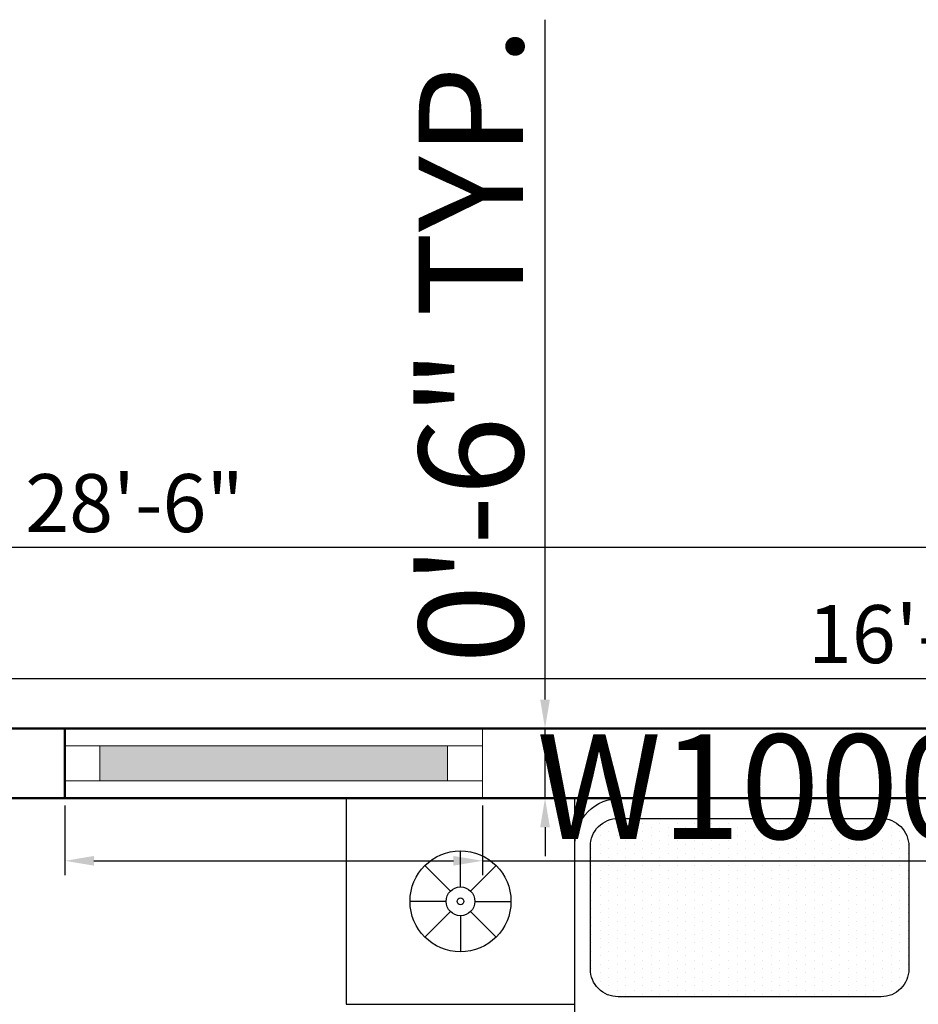
# Model space of a CAD drawing. Units: inches. Extents: x 3064 to 19385, y 846 to 15425.
# Tile 46 of 108: x 5352 to 5430, y 1368 to 1453. Entities that reach past the tile are written whole.
import ezdxf

# ---------------------------------------------------------------- set-up
doc = ezdxf.new("R2010")
doc.units = ezdxf.units.IN
for name, color, linetype, lineweight in [('A-ANNO-DIMS', 2, 'Continuous', 18), ('A-FLOR-FIXT', 9, 'Continuous', 18), ('A-GLAZ', 4, 'Continuous', 18), ('A-WALL', 7, 'Continuous', 50)]:
    doc.layers.add(name, color=color, linetype=linetype, lineweight=lineweight)
doc.layers.add('BLOCK', color=6, linetype='Continuous')
doc.styles.get("Standard").update_dxf_attribs({"font": 'arial.ttf'})
doc.dimstyles.new('ISO-25', dxfattribs={"dimtxt": 9, "dimasz": 2.5, "dimexe": 1.25, "dimexo": 0.625, "dimtad": 1, "dimdec": 1, "dimlunit": 3, "dimtxsty": 'Standard', "dimcen": 2.5, "dimadec": 0, "dimazin": 0, "dimtfac": 1, "dimtdec": 1, "dimtmove": 0, "dimatfit": 3, "dimfxl": 1, "dimarcsym": 0})

# ---------------------------------------------------------------- blocks, each defined once
blk = doc.blocks.new('*X7')
at = {"color": 0}
for p, q in [((266.25, 456.9375), (266.25, 456.9375)), ((266.4375, 457.03125), (266.4375, 457.03125)), ((266.625, 456.9375), (266.625, 456.9375)), ((266.8125, 457.03125), (266.8125, 457.03125)), ((267, 456.9375), (267, 456.9375)), ((267.1875, 457.03125), (267.1875, 457.03125)), ((267.375, 456.9375), (267.375, 456.9375)), ((267.5625, 457.03125), (267.5625, 457.03125)), ((267.75, 456.9375), (267.75, 456.9375)), ((267.9375, 457.03125), (267.9375, 457.03125)), ((268.125, 456.9375), (268.125, 456.9375)), ((268.3125, 457.03125), (268.3125, 457.03125)), ((268.5, 456.9375), (268.5, 456.9375)), ((268.6875, 457.03125), (268.6875, 457.03125)), ((268.875, 456.9375), (268.875, 456.9375)), ((269.0625, 457.03125), (269.0625, 457.03125)), ((269.25, 456.9375), (269.25, 456.9375)), ((269.4375, 457.03125), (269.4375, 457.03125)), ((269.625, 456.9375), (269.625, 456.9375)), ((269.8125, 457.03125), (269.8125, 457.03125)), ((270, 456.9375), (270, 456.9375)), ((270.1875, 457.03125), (270.1875, 457.03125)), ((270.375, 456.9375), (270.375, 456.9375)), ((270.5625, 457.03125), (270.5625, 457.03125)), ((270.75, 456.9375), (270.75, 456.9375)), ((270.9375, 457.03125), (270.9375, 457.03125)), ((271.125, 456.9375), (271.125, 456.9375)), ((271.3125, 457.03125), (271.3125, 457.03125)), ((271.5, 456.9375), (271.5, 456.9375)), ((271.6875, 457.03125), (271.6875, 457.03125)), ((271.875, 456.9375), (271.875, 456.9375)), ((272.0625, 457.03125), (272.0625, 457.03125)), ((272.25, 456.9375), (272.25, 456.9375)), ((266.0625, 456.84375), (266.0625, 456.84375)), ((266.0625, 456.65625), (266.0625, 456.65625)), ((266.25, 456.75), (266.25, 456.75)), ((266.4375, 456.84375), (266.4375, 456.84375)), ((266.4375, 456.65625), (266.4375, 456.65625)), ((266.625, 456.75), (266.625, 456.75)), ((266.8125, 456.84375), (266.8125, 456.84375)), ((266.8125, 456.65625), (266.8125, 456.65625)), ((267, 456.75), (267, 456.75)), ((267.1875, 456.84375), (267.1875, 456.84375)), ((267.1875, 456.65625), (267.1875, 456.65625)), ((267.375, 456.75), (267.375, 456.75)), ((267.5625, 456.84375), (267.5625, 456.84375)), ((267.5625, 456.65625), (267.5625, 456.65625)), ((267.75, 456.75), (267.75, 456.75)), ((267.9375, 456.84375), (267.9375, 456.84375)), ((267.9375, 456.65625), (267.9375, 456.65625)), ((268.125, 456.75), (268.125, 456.75)), ((268.3125, 456.84375), (268.3125, 456.84375)), ((268.3125, 456.65625), (268.3125, 456.65625)), ((268.5, 456.75), (268.5, 456.75)), ((268.6875, 456.84375), (268.6875, 456.84375)), ((268.6875, 456.65625), (268.6875, 456.65625)), ((268.875, 456.75), (268.875, 456.75)), ((269.0625, 456.84375), (269.0625, 456.84375)), ((269.0625, 456.65625), (269.0625, 456.65625)), ((269.25, 456.75), (269.25, 456.75)), ((269.4375, 456.84375), (269.4375, 456.84375)), ((269.4375, 456.65625), (269.4375, 456.65625)), ((269.625, 456.75), (269.625, 456.75)), ((269.8125, 456.84375), (269.8125, 456.84375)), ((269.8125, 456.65625), (269.8125, 456.65625)), ((270, 456.75), (270, 456.75)), ((270.1875, 456.84375), (270.1875, 456.84375)), ((270.1875, 456.65625), (270.1875, 456.65625)), ((270.375, 456.75), (270.375, 456.75)), ((270.5625, 456.84375), (270.5625, 456.84375)), ((270.5625, 456.65625), (270.5625, 456.65625)), ((270.75, 456.75), (270.75, 456.75)), ((270.9375, 456.84375), (270.9375, 456.84375)), ((270.9375, 456.65625), (270.9375, 456.65625)), ((271.125, 456.75), (271.125, 456.75)), ((271.3125, 456.84375), (271.3125, 456.84375)), ((271.3125, 456.65625), (271.3125, 456.65625)), ((271.5, 456.75), (271.5, 456.75)), ((271.6875, 456.84375), (271.6875, 456.84375)), ((271.6875, 456.65625), (271.6875, 456.65625)), ((271.875, 456.75), (271.875, 456.75)), ((272.0625, 456.84375), (272.0625, 456.84375)), ((272.0625, 456.65625), (272.0625, 456.65625)), ((272.25, 456.75), (272.25, 456.75)), ((272.4375, 456.84375), (272.4375, 456.84375)), ((272.4375, 456.65625), (272.4375, 456.65625)), ((272.625, 456.75), (272.625, 456.75)), ((265.875, 456.5625), (265.875, 456.5625)), ((266.0625, 456.46875), (266.0625, 456.46875)), ((266.25, 456.5625), (266.25, 456.5625)), ((266.4375, 456.46875), (266.4375, 456.46875)), ((266.625, 456.5625), (266.625, 456.5625)), ((266.8125, 456.46875), (266.8125, 456.46875)), ((267, 456.5625), (267, 456.5625)), ((267.1875, 456.46875), (267.1875, 456.46875)), ((267.375, 456.5625), (267.375, 456.5625)), ((267.5625, 456.46875), (267.5625, 456.46875)), ((267.75, 456.5625), (267.75, 456.5625)), ((267.9375, 456.46875), (267.9375, 456.46875)), ((268.125, 456.5625), (268.125, 456.5625)), ((268.3125, 456.46875), (268.3125, 456.46875)), ((268.5, 456.5625), (268.5, 456.5625)), ((268.6875, 456.46875), (268.6875, 456.46875)), ((268.875, 456.5625), (268.875, 456.5625)), ((269.0625, 456.46875), (269.0625, 456.46875)), ((269.25, 456.5625), (269.25, 456.5625)), ((269.4375, 456.46875), (269.4375, 456.46875)), ((269.625, 456.5625), (269.625, 456.5625)), ((269.8125, 456.46875), (269.8125, 456.46875)), ((270, 456.5625), (270, 456.5625)), ((270.1875, 456.46875), (270.1875, 456.46875)), ((270.375, 456.5625), (270.375, 456.5625)), ((270.5625, 456.46875), (270.5625, 456.46875)), ((270.75, 456.5625), (270.75, 456.5625)), ((270.9375, 456.46875), (270.9375, 456.46875)), ((271.125, 456.5625), (271.125, 456.5625)), ((271.3125, 456.46875), (271.3125, 456.46875)), ((271.5, 456.5625), (271.5, 456.5625)), ((271.6875, 456.46875), (271.6875, 456.46875)), ((271.875, 456.5625), (271.875, 456.5625)), ((272.0625, 456.46875), (272.0625, 456.46875)), ((272.25, 456.5625), (272.25, 456.5625)), ((272.4375, 456.46875), (272.4375, 456.46875)), ((272.625, 456.5625), (272.625, 456.5625)), ((272.8125, 456.46875), (272.8125, 456.46875)), ((265.875, 456.375), (265.875, 456.375)), ((266.0625, 456.28125), (266.0625, 456.28125)), ((266.25, 456.375), (266.25, 456.375)), ((266.4375, 456.28125), (266.4375, 456.28125)), ((266.625, 456.375), (266.625, 456.375)), ((266.8125, 456.28125), (266.8125, 456.28125)), ((267, 456.375), (267, 456.375)), ((267.1875, 456.28125), (267.1875, 456.28125)), ((267.375, 456.375), (267.375, 456.375)), ((267.5625, 456.28125), (267.5625, 456.28125)), ((267.75, 456.375), (267.75, 456.375)), ((267.9375, 456.28125), (267.9375, 456.28125)), ((268.125, 456.375), (268.125, 456.375)), ((268.3125, 456.28125), (268.3125, 456.28125)), ((268.5, 456.375), (268.5, 456.375)), ((268.6875, 456.28125), (268.6875, 456.28125)), ((268.875, 456.375), (268.875, 456.375)), ((269.0625, 456.28125), (269.0625, 456.28125)), ((269.25, 456.375), (269.25, 456.375)), ((269.4375, 456.28125), (269.4375, 456.28125)), ((269.625, 456.375), (269.625, 456.375)), ((269.8125, 456.28125), (269.8125, 456.28125)), ((270, 456.375), (270, 456.375)), ((270.1875, 456.28125), (270.1875, 456.28125)), ((270.375, 456.375), (270.375, 456.375)), ((270.5625, 456.28125), (270.5625, 456.28125)), ((270.75, 456.375), (270.75, 456.375)), ((270.9375, 456.28125), (270.9375, 456.28125)), ((271.125, 456.375), (271.125, 456.375)), ((271.3125, 456.28125), (271.3125, 456.28125)), ((271.5, 456.375), (271.5, 456.375)), ((271.6875, 456.28125), (271.6875, 456.28125)), ((271.875, 456.375), (271.875, 456.375)), ((272.0625, 456.28125), (272.0625, 456.28125)), ((272.25, 456.375), (272.25, 456.375)), ((272.4375, 456.28125), (272.4375, 456.28125)), ((272.625, 456.375), (272.625, 456.375)), ((272.8125, 456.28125), (272.8125, 456.28125)), ((265.875, 456.1875), (265.875, 456.1875)), ((265.875, 456), (265.875, 456)), ((266.0625, 456.09375), (266.0625, 456.09375)), ((266.25, 456.1875), (266.25, 456.1875)), ((266.25, 456), (266.25, 456)), ((266.4375, 456.09375), (266.4375, 456.09375)), ((266.625, 456.1875), (266.625, 456.1875)), ((266.625, 456), (266.625, 456)), ((266.8125, 456.09375), (266.8125, 456.09375)), ((267, 456.1875), (267, 456.1875)), ((267, 456), (267, 456)), ((267.1875, 456.09375), (267.1875, 456.09375)), ((267.375, 456.1875), (267.375, 456.1875)), ((267.375, 456), (267.375, 456)), ((267.5625, 456.09375), (267.5625, 456.09375)), ((267.75, 456.1875), (267.75, 456.1875)), ((267.75, 456), (267.75, 456)), ((267.9375, 456.09375), (267.9375, 456.09375)), ((268.125, 456.1875), (268.125, 456.1875)), ((268.125, 456), (268.125, 456)), ((268.3125, 456.09375), (268.3125, 456.09375)), ((268.5, 456.1875), (268.5, 456.1875)), ((268.5, 456), (268.5, 456)), ((268.6875, 456.09375), (268.6875, 456.09375)), ((268.875, 456.1875), (268.875, 456.1875)), ((268.875, 456), (268.875, 456)), ((269.0625, 456.09375), (269.0625, 456.09375)), ((269.25, 456.1875), (269.25, 456.1875)), ((269.25, 456), (269.25, 456)), ((269.4375, 456.09375), (269.4375, 456.09375)), ((269.625, 456.1875), (269.625, 456.1875)), ((269.625, 456), (269.625, 456)), ((269.8125, 456.09375), (269.8125, 456.09375)), ((270, 456.1875), (270, 456.1875)), ((270, 456), (270, 456)), ((270.1875, 456.09375), (270.1875, 456.09375)), ((270.375, 456.1875), (270.375, 456.1875)), ((270.375, 456), (270.375, 456)), ((270.5625, 456.09375), (270.5625, 456.09375)), ((270.75, 456.1875), (270.75, 456.1875)), ((270.75, 456), (270.75, 456)), ((270.9375, 456.09375), (270.9375, 456.09375)), ((271.125, 456.1875), (271.125, 456.1875)), ((271.125, 456), (271.125, 456)), ((271.3125, 456.09375), (271.3125, 456.09375)), ((271.5, 456.1875), (271.5, 456.1875)), ((271.5, 456), (271.5, 456)), ((271.6875, 456.09375), (271.6875, 456.09375)), ((271.875, 456.1875), (271.875, 456.1875)), ((271.875, 456), (271.875, 456)), ((272.0625, 456.09375), (272.0625, 456.09375)), ((272.25, 456.1875), (272.25, 456.1875)), ((272.25, 456), (272.25, 456)), ((272.4375, 456.09375), (272.4375, 456.09375)), ((272.625, 456.1875), (272.625, 456.1875)), ((272.625, 456), (272.625, 456)), ((272.8125, 456.09375), (272.8125, 456.09375)), ((265.875, 455.8125), (265.875, 455.8125)), ((266.0625, 455.90625), (266.0625, 455.90625)), ((266.25, 455.8125), (266.25, 455.8125)), ((266.4375, 455.90625), (266.4375, 455.90625)), ((266.625, 455.8125), (266.625, 455.8125)), ((266.8125, 455.90625), (266.8125, 455.90625)), ((267, 455.8125), (267, 455.8125)), ((267.1875, 455.90625), (267.1875, 455.90625)), ((267.375, 455.8125), (267.375, 455.8125)), ((267.5625, 455.90625), (267.5625, 455.90625)), ((267.75, 455.8125), (267.75, 455.8125)), ((267.9375, 455.90625), (267.9375, 455.90625)), ((268.125, 455.8125), (268.125, 455.8125)), ((268.3125, 455.90625), (268.3125, 455.90625)), ((268.5, 455.8125), (268.5, 455.8125)), ((268.6875, 455.90625), (268.6875, 455.90625)), ((268.875, 455.8125), (268.875, 455.8125)), ((269.0625, 455.90625), (269.0625, 455.90625)), ((269.25, 455.8125), (269.25, 455.8125)), ((269.4375, 455.90625), (269.4375, 455.90625)), ((269.625, 455.8125), (269.625, 455.8125)), ((269.8125, 455.90625), (269.8125, 455.90625)), ((270, 455.8125), (270, 455.8125)), ((270.1875, 455.90625), (270.1875, 455.90625)), ((270.375, 455.8125), (270.375, 455.8125)), ((270.5625, 455.90625), (270.5625, 455.90625)), ((270.75, 455.8125), (270.75, 455.8125)), ((270.9375, 455.90625), (270.9375, 455.90625)), ((271.125, 455.8125), (271.125, 455.8125)), ((271.3125, 455.90625), (271.3125, 455.90625)), ((271.5, 455.8125), (271.5, 455.8125)), ((271.6875, 455.90625), (271.6875, 455.90625)), ((271.875, 455.8125), (271.875, 455.8125)), ((272.0625, 455.90625), (272.0625, 455.90625)), ((272.25, 455.8125), (272.25, 455.8125)), ((272.4375, 455.90625), (272.4375, 455.90625)), ((272.625, 455.8125), (272.625, 455.8125)), ((272.8125, 455.90625), (272.8125, 455.90625)), ((265.875, 455.625), (265.875, 455.625)), ((266.0625, 455.71875), (266.0625, 455.71875)), ((266.25, 455.625), (266.25, 455.625)), ((266.4375, 455.71875), (266.4375, 455.71875)), ((266.625, 455.625), (266.625, 455.625)), ((266.8125, 455.71875), (266.8125, 455.71875)), ((267, 455.625), (267, 455.625)), ((267.1875, 455.71875), (267.1875, 455.71875)), ((267.375, 455.625), (267.375, 455.625)), ((267.5625, 455.71875), (267.5625, 455.71875)), ((267.75, 455.625), (267.75, 455.625)), ((267.9375, 455.71875), (267.9375, 455.71875)), ((268.125, 455.625), (268.125, 455.625)), ((268.3125, 455.71875), (268.3125, 455.71875)), ((268.5, 455.625), (268.5, 455.625)), ((268.6875, 455.71875), (268.6875, 455.71875)), ((268.875, 455.625), (268.875, 455.625)), ((269.0625, 455.71875), (269.0625, 455.71875)), ((269.25, 455.625), (269.25, 455.625)), ((269.4375, 455.71875), (269.4375, 455.71875)), ((269.625, 455.625), (269.625, 455.625)), ((269.8125, 455.71875), (269.8125, 455.71875)), ((270, 455.625), (270, 455.625)), ((270.1875, 455.71875), (270.1875, 455.71875)), ((270.375, 455.625), (270.375, 455.625)), ((270.5625, 455.71875), (270.5625, 455.71875)), ((270.75, 455.625), (270.75, 455.625)), ((270.9375, 455.71875), (270.9375, 455.71875)), ((271.125, 455.625), (271.125, 455.625)), ((271.3125, 455.71875), (271.3125, 455.71875)), ((271.5, 455.625), (271.5, 455.625)), ((271.6875, 455.71875), (271.6875, 455.71875)), ((271.875, 455.625), (271.875, 455.625)), ((272.0625, 455.71875), (272.0625, 455.71875)), ((272.25, 455.625), (272.25, 455.625)), ((272.4375, 455.71875), (272.4375, 455.71875)), ((272.625, 455.625), (272.625, 455.625)), ((272.8125, 455.71875), (272.8125, 455.71875)), ((265.875, 455.4375), (265.875, 455.4375)), ((266.0625, 455.53125), (266.0625, 455.53125)), ((266.0625, 455.34375), (266.0625, 455.34375)), ((266.25, 455.4375), (266.25, 455.4375)), ((266.4375, 455.53125), (266.4375, 455.53125)), ((266.4375, 455.34375), (266.4375, 455.34375)), ((266.625, 455.4375), (266.625, 455.4375)), ((266.8125, 455.53125), (266.8125, 455.53125)), ((266.8125, 455.34375), (266.8125, 455.34375)), ((267, 455.4375), (267, 455.4375)), ((267.1875, 455.53125), (267.1875, 455.53125)), ((267.1875, 455.34375), (267.1875, 455.34375)), ((267.375, 455.4375), (267.375, 455.4375)), ((267.5625, 455.53125), (267.5625, 455.53125)), ((267.5625, 455.34375), (267.5625, 455.34375)), ((267.75, 455.4375), (267.75, 455.4375)), ((267.9375, 455.53125), (267.9375, 455.53125)), ((267.9375, 455.34375), (267.9375, 455.34375)), ((268.125, 455.4375), (268.125, 455.4375)), ((268.3125, 455.53125), (268.3125, 455.53125)), ((268.3125, 455.34375), (268.3125, 455.34375)), ((268.5, 455.4375), (268.5, 455.4375)), ((268.6875, 455.53125), (268.6875, 455.53125)), ((268.6875, 455.34375), (268.6875, 455.34375)), ((268.875, 455.4375), (268.875, 455.4375)), ((269.0625, 455.53125), (269.0625, 455.53125)), ((269.0625, 455.34375), (269.0625, 455.34375)), ((269.25, 455.4375), (269.25, 455.4375)), ((269.4375, 455.53125), (269.4375, 455.53125)), ((269.4375, 455.34375), (269.4375, 455.34375)), ((269.625, 455.4375), (269.625, 455.4375)), ((269.8125, 455.53125), (269.8125, 455.53125)), ((269.8125, 455.34375), (269.8125, 455.34375)), ((270, 455.4375), (270, 455.4375)), ((270.1875, 455.53125), (270.1875, 455.53125)), ((270.1875, 455.34375), (270.1875, 455.34375)), ((270.375, 455.4375), (270.375, 455.4375)), ((270.5625, 455.53125), (270.5625, 455.53125)), ((270.5625, 455.34375), (270.5625, 455.34375)), ((270.75, 455.4375), (270.75, 455.4375)), ((270.9375, 455.53125), (270.9375, 455.53125)), ((270.9375, 455.34375), (270.9375, 455.34375)), ((271.125, 455.4375), (271.125, 455.4375)), ((271.3125, 455.53125), (271.3125, 455.53125)), ((271.3125, 455.34375), (271.3125, 455.34375)), ((271.5, 455.4375), (271.5, 455.4375)), ((271.6875, 455.53125), (271.6875, 455.53125)), ((271.6875, 455.34375), (271.6875, 455.34375)), ((271.875, 455.4375), (271.875, 455.4375)), ((272.0625, 455.53125), (272.0625, 455.53125)), ((272.0625, 455.34375), (272.0625, 455.34375)), ((272.25, 455.4375), (272.25, 455.4375)), ((272.4375, 455.53125), (272.4375, 455.53125)), ((272.4375, 455.34375), (272.4375, 455.34375)), ((272.625, 455.4375), (272.625, 455.4375)), ((272.8125, 455.53125), (272.8125, 455.53125)), ((272.8125, 455.34375), (272.8125, 455.34375)), ((265.875, 455.25), (265.875, 455.25)), ((266.0625, 455.15625), (266.0625, 455.15625)), ((266.25, 455.25), (266.25, 455.25)), ((266.4375, 455.15625), (266.4375, 455.15625)), ((266.625, 455.25), (266.625, 455.25)), ((266.8125, 455.15625), (266.8125, 455.15625)), ((267, 455.25), (267, 455.25)), ((267.1875, 455.15625), (267.1875, 455.15625)), ((267.375, 455.25), (267.375, 455.25)), ((267.5625, 455.15625), (267.5625, 455.15625)), ((267.75, 455.25), (267.75, 455.25)), ((267.9375, 455.15625), (267.9375, 455.15625)), ((268.125, 455.25), (268.125, 455.25)), ((268.3125, 455.15625), (268.3125, 455.15625)), ((268.5, 455.25), (268.5, 455.25)), ((268.6875, 455.15625), (268.6875, 455.15625)), ((268.875, 455.25), (268.875, 455.25)), ((269.0625, 455.15625), (269.0625, 455.15625)), ((269.25, 455.25), (269.25, 455.25)), ((269.4375, 455.15625), (269.4375, 455.15625)), ((269.625, 455.25), (269.625, 455.25)), ((269.8125, 455.15625), (269.8125, 455.15625)), ((270, 455.25), (270, 455.25)), ((270.1875, 455.15625), (270.1875, 455.15625)), ((270.375, 455.25), (270.375, 455.25)), ((270.5625, 455.15625), (270.5625, 455.15625)), ((270.75, 455.25), (270.75, 455.25)), ((270.9375, 455.15625), (270.9375, 455.15625)), ((271.125, 455.25), (271.125, 455.25)), ((271.3125, 455.15625), (271.3125, 455.15625)), ((271.5, 455.25), (271.5, 455.25)), ((271.6875, 455.15625), (271.6875, 455.15625)), ((271.875, 455.25), (271.875, 455.25)), ((272.0625, 455.15625), (272.0625, 455.15625)), ((272.25, 455.25), (272.25, 455.25)), ((272.4375, 455.15625), (272.4375, 455.15625)), ((272.625, 455.25), (272.625, 455.25)), ((272.8125, 455.15625), (272.8125, 455.15625)), ((265.875, 455.0625), (265.875, 455.0625)), ((266.0625, 454.96875), (266.0625, 454.96875)), ((266.25, 455.0625), (266.25, 455.0625)), ((266.4375, 454.96875), (266.4375, 454.96875)), ((266.625, 455.0625), (266.625, 455.0625)), ((266.8125, 454.96875), (266.8125, 454.96875)), ((267, 455.0625), (267, 455.0625)), ((267.1875, 454.96875), (267.1875, 454.96875)), ((267.375, 455.0625), (267.375, 455.0625)), ((267.5625, 454.96875), (267.5625, 454.96875)), ((267.75, 455.0625), (267.75, 455.0625)), ((267.9375, 454.96875), (267.9375, 454.96875)), ((268.125, 455.0625), (268.125, 455.0625)), ((268.3125, 454.96875), (268.3125, 454.96875)), ((268.5, 455.0625), (268.5, 455.0625)), ((268.6875, 454.96875), (268.6875, 454.96875)), ((268.875, 455.0625), (268.875, 455.0625)), ((269.0625, 454.96875), (269.0625, 454.96875)), ((269.25, 455.0625), (269.25, 455.0625)), ((269.4375, 454.96875), (269.4375, 454.96875)), ((269.625, 455.0625), (269.625, 455.0625)), ((269.8125, 454.96875), (269.8125, 454.96875)), ((270, 455.0625), (270, 455.0625)), ((270.1875, 454.96875), (270.1875, 454.96875)), ((270.375, 455.0625), (270.375, 455.0625)), ((270.5625, 454.96875), (270.5625, 454.96875)), ((270.75, 455.0625), (270.75, 455.0625)), ((270.9375, 454.96875), (270.9375, 454.96875)), ((271.125, 455.0625), (271.125, 455.0625)), ((271.3125, 454.96875), (271.3125, 454.96875)), ((271.5, 455.0625), (271.5, 455.0625)), ((271.6875, 454.96875), (271.6875, 454.96875)), ((271.875, 455.0625), (271.875, 455.0625)), ((272.0625, 454.96875), (272.0625, 454.96875)), ((272.25, 455.0625), (272.25, 455.0625)), ((272.4375, 454.96875), (272.4375, 454.96875)), ((272.625, 455.0625), (272.625, 455.0625)), ((272.8125, 454.96875), (272.8125, 454.96875)), ((265.875, 454.875), (265.875, 454.875)), ((266.0625, 454.78125), (266.0625, 454.78125)), ((266.25, 454.875), (266.25, 454.875)), ((266.4375, 454.78125), (266.4375, 454.78125)), ((266.625, 454.875), (266.625, 454.875)), ((266.8125, 454.78125), (266.8125, 454.78125)), ((267, 454.875), (267, 454.875)), ((267.1875, 454.78125), (267.1875, 454.78125)), ((267.375, 454.875), (267.375, 454.875)), ((267.5625, 454.78125), (267.5625, 454.78125)), ((267.75, 454.875), (267.75, 454.875)), ((267.9375, 454.78125), (267.9375, 454.78125)), ((268.125, 454.875), (268.125, 454.875)), ((268.3125, 454.78125), (268.3125, 454.78125)), ((268.5, 454.875), (268.5, 454.875)), ((268.6875, 454.78125), (268.6875, 454.78125)), ((268.875, 454.875), (268.875, 454.875)), ((269.0625, 454.78125), (269.0625, 454.78125)), ((269.25, 454.875), (269.25, 454.875)), ((269.4375, 454.78125), (269.4375, 454.78125)), ((269.625, 454.875), (269.625, 454.875)), ((269.8125, 454.78125), (269.8125, 454.78125)), ((270, 454.875), (270, 454.875)), ((270.1875, 454.78125), (270.1875, 454.78125)), ((270.375, 454.875), (270.375, 454.875)), ((270.5625, 454.78125), (270.5625, 454.78125)), ((270.75, 454.875), (270.75, 454.875)), ((270.9375, 454.78125), (270.9375, 454.78125)), ((271.125, 454.875), (271.125, 454.875)), ((271.3125, 454.78125), (271.3125, 454.78125)), ((271.5, 454.875), (271.5, 454.875)), ((271.6875, 454.78125), (271.6875, 454.78125)), ((271.875, 454.875), (271.875, 454.875)), ((272.0625, 454.78125), (272.0625, 454.78125)), ((272.25, 454.875), (272.25, 454.875)), ((272.4375, 454.78125), (272.4375, 454.78125)), ((272.625, 454.875), (272.625, 454.875)), ((272.8125, 454.78125), (272.8125, 454.78125)), ((265.875, 454.6875), (265.875, 454.6875)), ((265.875, 454.5), (265.875, 454.5)), ((266.0625, 454.59375), (266.0625, 454.59375)), ((266.25, 454.6875), (266.25, 454.6875)), ((266.25, 454.5), (266.25, 454.5)), ((266.4375, 454.59375), (266.4375, 454.59375)), ((266.625, 454.6875), (266.625, 454.6875)), ((266.625, 454.5), (266.625, 454.5)), ((266.8125, 454.59375), (266.8125, 454.59375)), ((267, 454.6875), (267, 454.6875)), ((267, 454.5), (267, 454.5)), ((267.1875, 454.59375), (267.1875, 454.59375)), ((267.375, 454.6875), (267.375, 454.6875)), ((267.375, 454.5), (267.375, 454.5)), ((267.5625, 454.59375), (267.5625, 454.59375)), ((267.75, 454.6875), (267.75, 454.6875)), ((267.75, 454.5), (267.75, 454.5)), ((267.9375, 454.59375), (267.9375, 454.59375)), ((268.125, 454.6875), (268.125, 454.6875)), ((268.125, 454.5), (268.125, 454.5)), ((268.3125, 454.59375), (268.3125, 454.59375)), ((268.5, 454.6875), (268.5, 454.6875)), ((268.5, 454.5), (268.5, 454.5)), ((268.6875, 454.59375), (268.6875, 454.59375)), ((268.875, 454.6875), (268.875, 454.6875)), ((268.875, 454.5), (268.875, 454.5)), ((269.0625, 454.59375), (269.0625, 454.59375)), ((269.25, 454.6875), (269.25, 454.6875)), ((269.25, 454.5), (269.25, 454.5)), ((269.4375, 454.59375), (269.4375, 454.59375)), ((269.625, 454.6875), (269.625, 454.6875)), ((269.625, 454.5), (269.625, 454.5)), ((269.8125, 454.59375), (269.8125, 454.59375)), ((270, 454.6875), (270, 454.6875)), ((270, 454.5), (270, 454.5)), ((270.1875, 454.59375), (270.1875, 454.59375)), ((270.375, 454.6875), (270.375, 454.6875)), ((270.375, 454.5), (270.375, 454.5)), ((270.5625, 454.59375), (270.5625, 454.59375)), ((270.75, 454.6875), (270.75, 454.6875)), ((270.75, 454.5), (270.75, 454.5)), ((270.9375, 454.59375), (270.9375, 454.59375)), ((271.125, 454.6875), (271.125, 454.6875)), ((271.125, 454.5), (271.125, 454.5)), ((271.3125, 454.59375), (271.3125, 454.59375)), ((271.5, 454.6875), (271.5, 454.6875)), ((271.5, 454.5), (271.5, 454.5)), ((271.6875, 454.59375), (271.6875, 454.59375)), ((271.875, 454.6875), (271.875, 454.6875)), ((271.875, 454.5), (271.875, 454.5)), ((272.0625, 454.59375), (272.0625, 454.59375)), ((272.25, 454.6875), (272.25, 454.6875)), ((272.25, 454.5), (272.25, 454.5)), ((272.4375, 454.59375), (272.4375, 454.59375)), ((272.625, 454.6875), (272.625, 454.6875)), ((272.625, 454.5), (272.625, 454.5)), ((272.8125, 454.59375), (272.8125, 454.59375)), ((265.875, 454.3125), (265.875, 454.3125)), ((266.0625, 454.40625), (266.0625, 454.40625)), ((266.25, 454.3125), (266.25, 454.3125)), ((266.4375, 454.40625), (266.4375, 454.40625)), ((266.625, 454.3125), (266.625, 454.3125)), ((266.8125, 454.40625), (266.8125, 454.40625)), ((267, 454.3125), (267, 454.3125)), ((267.1875, 454.40625), (267.1875, 454.40625)), ((267.375, 454.3125), (267.375, 454.3125)), ((267.5625, 454.40625), (267.5625, 454.40625)), ((267.75, 454.3125), (267.75, 454.3125)), ((267.9375, 454.40625), (267.9375, 454.40625)), ((268.125, 454.3125), (268.125, 454.3125)), ((268.3125, 454.40625), (268.3125, 454.40625)), ((268.5, 454.3125), (268.5, 454.3125)), ((268.6875, 454.40625), (268.6875, 454.40625)), ((268.875, 454.3125), (268.875, 454.3125)), ((269.0625, 454.40625), (269.0625, 454.40625)), ((269.25, 454.3125), (269.25, 454.3125)), ((269.4375, 454.40625), (269.4375, 454.40625)), ((269.625, 454.3125), (269.625, 454.3125)), ((269.8125, 454.40625), (269.8125, 454.40625)), ((270, 454.3125), (270, 454.3125)), ((270.1875, 454.40625), (270.1875, 454.40625)), ((270.375, 454.3125), (270.375, 454.3125)), ((270.5625, 454.40625), (270.5625, 454.40625)), ((270.75, 454.3125), (270.75, 454.3125)), ((270.9375, 454.40625), (270.9375, 454.40625)), ((271.125, 454.3125), (271.125, 454.3125)), ((271.3125, 454.40625), (271.3125, 454.40625)), ((271.5, 454.3125), (271.5, 454.3125)), ((271.6875, 454.40625), (271.6875, 454.40625)), ((271.875, 454.3125), (271.875, 454.3125)), ((272.0625, 454.40625), (272.0625, 454.40625)), ((272.25, 454.3125), (272.25, 454.3125)), ((272.4375, 454.40625), (272.4375, 454.40625)), ((272.625, 454.3125), (272.625, 454.3125)), ((272.8125, 454.40625), (272.8125, 454.40625)), ((265.875, 454.125), (265.875, 454.125)), ((266.0625, 454.21875), (266.0625, 454.21875)), ((266.25, 454.125), (266.25, 454.125)), ((266.4375, 454.21875), (266.4375, 454.21875)), ((266.625, 454.125), (266.625, 454.125)), ((266.8125, 454.21875), (266.8125, 454.21875)), ((267, 454.125), (267, 454.125)), ((267.1875, 454.21875), (267.1875, 454.21875)), ((267.375, 454.125), (267.375, 454.125)), ((267.5625, 454.21875), (267.5625, 454.21875)), ((267.75, 454.125), (267.75, 454.125)), ((267.9375, 454.21875), (267.9375, 454.21875)), ((268.125, 454.125), (268.125, 454.125)), ((268.3125, 454.21875), (268.3125, 454.21875)), ((268.5, 454.125), (268.5, 454.125)), ((268.6875, 454.21875), (268.6875, 454.21875)), ((268.875, 454.125), (268.875, 454.125)), ((269.0625, 454.21875), (269.0625, 454.21875)), ((269.25, 454.125), (269.25, 454.125)), ((269.4375, 454.21875), (269.4375, 454.21875)), ((269.625, 454.125), (269.625, 454.125)), ((269.8125, 454.21875), (269.8125, 454.21875)), ((270, 454.125), (270, 454.125)), ((270.1875, 454.21875), (270.1875, 454.21875)), ((270.375, 454.125), (270.375, 454.125)), ((270.5625, 454.21875), (270.5625, 454.21875)), ((270.75, 454.125), (270.75, 454.125)), ((270.9375, 454.21875), (270.9375, 454.21875)), ((271.125, 454.125), (271.125, 454.125)), ((271.3125, 454.21875), (271.3125, 454.21875)), ((271.5, 454.125), (271.5, 454.125)), ((271.6875, 454.21875), (271.6875, 454.21875)), ((271.875, 454.125), (271.875, 454.125)), ((272.0625, 454.21875), (272.0625, 454.21875)), ((272.25, 454.125), (272.25, 454.125)), ((272.4375, 454.21875), (272.4375, 454.21875)), ((272.625, 454.125), (272.625, 454.125)), ((272.8125, 454.21875), (272.8125, 454.21875)), ((265.875, 453.9375), (265.875, 453.9375)), ((266.0625, 454.03125), (266.0625, 454.03125)), ((266.0625, 453.84375), (266.0625, 453.84375)), ((266.25, 453.9375), (266.25, 453.9375)), ((266.4375, 454.03125), (266.4375, 454.03125)), ((266.4375, 453.84375), (266.4375, 453.84375)), ((266.625, 453.9375), (266.625, 453.9375)), ((266.8125, 454.03125), (266.8125, 454.03125)), ((266.8125, 453.84375), (266.8125, 453.84375)), ((267, 453.9375), (267, 453.9375)), ((267.1875, 454.03125), (267.1875, 454.03125)), ((267.1875, 453.84375), (267.1875, 453.84375)), ((267.375, 453.9375), (267.375, 453.9375)), ((267.5625, 454.03125), (267.5625, 454.03125)), ((267.5625, 453.84375), (267.5625, 453.84375)), ((267.75, 453.9375), (267.75, 453.9375)), ((267.9375, 454.03125), (267.9375, 454.03125)), ((267.9375, 453.84375), (267.9375, 453.84375)), ((268.125, 453.9375), (268.125, 453.9375)), ((268.3125, 454.03125), (268.3125, 454.03125)), ((268.3125, 453.84375), (268.3125, 453.84375)), ((268.5, 453.9375), (268.5, 453.9375)), ((268.6875, 454.03125), (268.6875, 454.03125)), ((268.6875, 453.84375), (268.6875, 453.84375)), ((268.875, 453.9375), (268.875, 453.9375)), ((269.0625, 454.03125), (269.0625, 454.03125)), ((269.0625, 453.84375), (269.0625, 453.84375)), ((269.25, 453.9375), (269.25, 453.9375)), ((269.4375, 454.03125), (269.4375, 454.03125)), ((269.4375, 453.84375), (269.4375, 453.84375)), ((269.625, 453.9375), (269.625, 453.9375)), ((269.8125, 454.03125), (269.8125, 454.03125)), ((269.8125, 453.84375), (269.8125, 453.84375)), ((270, 453.9375), (270, 453.9375)), ((270.1875, 454.03125), (270.1875, 454.03125)), ((270.1875, 453.84375), (270.1875, 453.84375)), ((270.375, 453.9375), (270.375, 453.9375)), ((270.5625, 454.03125), (270.5625, 454.03125)), ((270.5625, 453.84375), (270.5625, 453.84375)), ((270.75, 453.9375), (270.75, 453.9375)), ((270.9375, 454.03125), (270.9375, 454.03125)), ((270.9375, 453.84375), (270.9375, 453.84375)), ((271.125, 453.9375), (271.125, 453.9375)), ((271.3125, 454.03125), (271.3125, 454.03125)), ((271.3125, 453.84375), (271.3125, 453.84375)), ((271.5, 453.9375), (271.5, 453.9375)), ((271.6875, 454.03125), (271.6875, 454.03125)), ((271.6875, 453.84375), (271.6875, 453.84375)), ((271.875, 453.9375), (271.875, 453.9375)), ((272.0625, 454.03125), (272.0625, 454.03125)), ((272.0625, 453.84375), (272.0625, 453.84375)), ((272.25, 453.9375), (272.25, 453.9375)), ((272.4375, 454.03125), (272.4375, 454.03125)), ((272.4375, 453.84375), (272.4375, 453.84375)), ((272.625, 453.9375), (272.625, 453.9375)), ((272.8125, 454.03125), (272.8125, 454.03125)), ((272.8125, 453.84375), (272.8125, 453.84375)), ((265.875, 453.75), (265.875, 453.75)), ((266.0625, 453.65625), (266.0625, 453.65625)), ((266.25, 453.75), (266.25, 453.75)), ((266.4375, 453.65625), (266.4375, 453.65625)), ((266.625, 453.75), (266.625, 453.75)), ((266.8125, 453.65625), (266.8125, 453.65625)), ((267, 453.75), (267, 453.75)), ((267.1875, 453.65625), (267.1875, 453.65625)), ((267.375, 453.75), (267.375, 453.75)), ((267.5625, 453.65625), (267.5625, 453.65625)), ((267.75, 453.75), (267.75, 453.75)), ((267.9375, 453.65625), (267.9375, 453.65625)), ((268.125, 453.75), (268.125, 453.75)), ((268.3125, 453.65625), (268.3125, 453.65625)), ((268.5, 453.75), (268.5, 453.75)), ((268.6875, 453.65625), (268.6875, 453.65625)), ((268.875, 453.75), (268.875, 453.75)), ((269.0625, 453.65625), (269.0625, 453.65625)), ((269.25, 453.75), (269.25, 453.75)), ((269.4375, 453.65625), (269.4375, 453.65625)), ((269.625, 453.75), (269.625, 453.75)), ((269.8125, 453.65625), (269.8125, 453.65625)), ((270, 453.75), (270, 453.75)), ((270.1875, 453.65625), (270.1875, 453.65625)), ((270.375, 453.75), (270.375, 453.75)), ((270.5625, 453.65625), (270.5625, 453.65625)), ((270.75, 453.75), (270.75, 453.75)), ((270.9375, 453.65625), (270.9375, 453.65625)), ((271.125, 453.75), (271.125, 453.75)), ((271.3125, 453.65625), (271.3125, 453.65625)), ((271.5, 453.75), (271.5, 453.75)), ((271.6875, 453.65625), (271.6875, 453.65625)), ((271.875, 453.75), (271.875, 453.75)), ((272.0625, 453.65625), (272.0625, 453.65625)), ((272.25, 453.75), (272.25, 453.75)), ((272.4375, 453.65625), (272.4375, 453.65625)), ((272.625, 453.75), (272.625, 453.75)), ((272.8125, 453.65625), (272.8125, 453.65625)), ((266.0625, 453.46875), (266.0625, 453.46875)), ((266.25, 453.5625), (266.25, 453.5625)), ((266.4375, 453.46875), (266.4375, 453.46875)), ((266.625, 453.5625), (266.625, 453.5625)), ((266.8125, 453.46875), (266.8125, 453.46875)), ((267, 453.5625), (267, 453.5625)), ((267.1875, 453.46875), (267.1875, 453.46875)), ((267.375, 453.5625), (267.375, 453.5625)), ((267.5625, 453.46875), (267.5625, 453.46875)), ((267.75, 453.5625), (267.75, 453.5625)), ((267.9375, 453.46875), (267.9375, 453.46875)), ((268.125, 453.5625), (268.125, 453.5625)), ((268.3125, 453.46875), (268.3125, 453.46875)), ((268.5, 453.5625), (268.5, 453.5625)), ((268.6875, 453.46875), (268.6875, 453.46875)), ((268.875, 453.5625), (268.875, 453.5625)), ((269.0625, 453.46875), (269.0625, 453.46875)), ((269.25, 453.5625), (269.25, 453.5625)), ((269.4375, 453.46875), (269.4375, 453.46875)), ((269.625, 453.5625), (269.625, 453.5625)), ((269.8125, 453.46875), (269.8125, 453.46875)), ((270, 453.5625), (270, 453.5625)), ((270.1875, 453.46875), (270.1875, 453.46875)), ((270.375, 453.5625), (270.375, 453.5625)), ((270.5625, 453.46875), (270.5625, 453.46875)), ((270.75, 453.5625), (270.75, 453.5625)), ((270.9375, 453.46875), (270.9375, 453.46875)), ((271.125, 453.5625), (271.125, 453.5625)), ((271.3125, 453.46875), (271.3125, 453.46875)), ((271.5, 453.5625), (271.5, 453.5625)), ((271.6875, 453.46875), (271.6875, 453.46875)), ((271.875, 453.5625), (271.875, 453.5625)), ((272.0625, 453.46875), (272.0625, 453.46875)), ((272.25, 453.5625), (272.25, 453.5625)), ((272.4375, 453.46875), (272.4375, 453.46875)), ((272.625, 453.5625), (272.625, 453.5625)), ((266.0625, 453.28125), (266.0625, 453.28125)), ((266.25, 453.375), (266.25, 453.375)), ((266.25, 453.1875), (266.25, 453.1875)), ((266.4375, 453.28125), (266.4375, 453.28125)), ((266.625, 453.375), (266.625, 453.375)), ((266.625, 453.1875), (266.625, 453.1875)), ((266.8125, 453.28125), (266.8125, 453.28125)), ((267, 453.375), (267, 453.375)), ((267, 453.1875), (267, 453.1875)), ((267.1875, 453.28125), (267.1875, 453.28125)), ((267.375, 453.375), (267.375, 453.375)), ((267.375, 453.1875), (267.375, 453.1875)), ((267.5625, 453.28125), (267.5625, 453.28125)), ((267.75, 453.375), (267.75, 453.375)), ((267.75, 453.1875), (267.75, 453.1875)), ((267.9375, 453.28125), (267.9375, 453.28125)), ((268.125, 453.375), (268.125, 453.375)), ((268.125, 453.1875), (268.125, 453.1875)), ((268.3125, 453.28125), (268.3125, 453.28125)), ((268.5, 453.375), (268.5, 453.375)), ((268.5, 453.1875), (268.5, 453.1875)), ((268.6875, 453.28125), (268.6875, 453.28125)), ((268.875, 453.375), (268.875, 453.375)), ((268.875, 453.1875), (268.875, 453.1875)), ((269.0625, 453.28125), (269.0625, 453.28125)), ((269.25, 453.375), (269.25, 453.375)), ((269.25, 453.1875), (269.25, 453.1875)), ((269.4375, 453.28125), (269.4375, 453.28125)), ((269.625, 453.375), (269.625, 453.375)), ((269.625, 453.1875), (269.625, 453.1875)), ((269.8125, 453.28125), (269.8125, 453.28125)), ((270, 453.375), (270, 453.375)), ((270, 453.1875), (270, 453.1875)), ((270.1875, 453.28125), (270.1875, 453.28125)), ((270.375, 453.375), (270.375, 453.375)), ((270.375, 453.1875), (270.375, 453.1875)), ((270.5625, 453.28125), (270.5625, 453.28125)), ((270.75, 453.375), (270.75, 453.375)), ((270.75, 453.1875), (270.75, 453.1875)), ((270.9375, 453.28125), (270.9375, 453.28125)), ((271.125, 453.375), (271.125, 453.375)), ((271.125, 453.1875), (271.125, 453.1875)), ((271.3125, 453.28125), (271.3125, 453.28125)), ((271.5, 453.375), (271.5, 453.375)), ((271.5, 453.1875), (271.5, 453.1875)), ((271.6875, 453.28125), (271.6875, 453.28125)), ((271.875, 453.375), (271.875, 453.375)), ((271.875, 453.1875), (271.875, 453.1875)), ((272.0625, 453.28125), (272.0625, 453.28125)), ((272.25, 453.375), (272.25, 453.375)), ((272.25, 453.1875), (272.25, 453.1875)), ((272.4375, 453.28125), (272.4375, 453.28125)), ((272.625, 453.375), (272.625, 453.375))]:
    blk.add_line(p, q, dxfattribs=at)
blk = doc.blocks.new('A$C52E67D0D')
at = {"layer": 'BLOCK'}
for p, q in [((250.5, 1605.5), (250.5, 1684.7)), ((228.3, 1596.3), (172.3, 1652.3)), ((272.7, 1596.3), (328.7, 1652.3)), ((219.1, 1574.1), (139.9, 1574.1)), ((281.9, 1574.1), (361.1, 1574.1)), ((228.3, 1551.9), (172.3, 1495.9)), ((250.5, 1542.8), (250.5, 1463.5)), ((272.7, 1551.9), (328.7, 1495.9))]:
    blk.add_line(p, q, dxfattribs=at)
blk.add_lwpolyline([(501, 1348.6), (501, 1799.6), (0, 1799.6), (0, 1348.6)], close=True, dxfattribs=at)
for points in [[(1901, 0), (601, 0, -0.414214), (501, 100), (501, 1700, -0.414214), (601, 1800), (1901, 1800, -0.414214), (2001, 1700), (2001, 100, -0.414214)], [(1171.8, 1365.1), (595.8, 1365.1, -0.414214), (535, 1425.9), (535, 1694.8, -0.414214), (595.8, 1755.7), (1171.8, 1755.7, -0.414214), (1232.6, 1694.8), (1232.6, 1425.9, -0.414214)]]:
    blk.add_lwpolyline(points, format="xyb", close=True, dxfattribs=at)
for radius in [110.6, 31.4, 7.46]:
    blk.add_circle((250.5, 1574.1), radius, dxfattribs=at)
blk.add_arc((1888.6, -1664.5), 3015.3, 87.8642, 117.4001, dxfattribs=at)
at = {"layer": 'BLOCK', "xscale": 100, "yscale": 100, "zscale": 100}
blk.add_blockref('*X7', (-26050, -43948.2), dxfattribs=at)
blk = doc.blocks.new('*D92')
at = {"layer": 'A-ANNO-DIMS', "color": 0, "lineweight": -2, "transparency": 16777216}
for p, q in [((5332.017, 1392.721), (5332.017, 1397.658)), ((5527.017, 1392.721), (5527.017, 1397.658)), ((5334.517, 1396.408), (5524.517, 1396.408))]:
    blk.add_line(p, q, dxfattribs=at)
at = {"layer": 'A-ANNO-DIMS', "color": 0, "transparency": 16777216}
for points in [[(5334.517, 1396.825), (5334.517, 1395.992), (5332.017, 1396.408)], [(5524.517, 1396.825), (5524.517, 1395.992), (5527.017, 1396.408)]]:
    blk.add_solid(points, dxfattribs=at)
at = {"layer": 'Defpoints', "color": 0, "transparency": 16777216}
for p in [(5527.017, 1396.408), (5332.017, 1392.096), (5527.017, 1392.096)]:
    blk.add_point(p, dxfattribs=at)
at = {"layer": 'A-ANNO-DIMS', "color": 0, "transparency": 16777216, "insert": (5429.517, 1399.588), "char_height": 5, "attachment_point": 5}
blk.add_mtext('16\'-3"', dxfattribs=at)
blk = doc.blocks.new('*D94')
at = {"layer": 'A-ANNO-DIMS', "color": 0, "lineweight": -2, "transparency": 16777216}
for p, q in [((5191.017, 1392.721), (5191.017, 1408.956)), ((5533.017, 1392.721), (5533.017, 1408.956)), ((5530.517, 1407.706), (5193.517, 1407.706))]:
    blk.add_line(p, q, dxfattribs=at)
at = {"layer": 'A-ANNO-DIMS', "color": 0, "transparency": 16777216}
for points in [[(5193.517, 1408.122), (5193.517, 1407.289), (5191.017, 1407.706)], [(5530.517, 1408.122), (5530.517, 1407.289), (5533.017, 1407.706)]]:
    blk.add_solid(points, dxfattribs=at)
at = {"layer": 'Defpoints', "color": 0, "transparency": 16777216}
for p in [(5191.017, 1407.706), (5191.017, 1392.096), (5533.017, 1392.096)]:
    blk.add_point(p, dxfattribs=at)
at = {"layer": 'A-ANNO-DIMS', "color": 0, "transparency": 16777216, "insert": (5362.017, 1410.884), "char_height": 5, "attachment_point": 5}
blk.add_mtext('28\'-6"', dxfattribs=at)
blk = doc.blocks.new('WIN-1000-B')
h = blk.add_hatch(color=256)
h.dxf.hatch_style = 1
h.paths.add_polyline_path([(33, 1.5), (33, 4.5), (3, 4.5), (3, 1.5)])
for p, q in [((36, 6), (36, 0)), ((3, 4.5), (33, 4.5)), ((3, 1.5), (33, 1.5))]:
    blk.add_line(p, q)
for points in [[(3, 1.5), (0, 1.5), (0, 4.5), (3, 4.5)], [(36, 1.5), (33, 1.5), (33, 4.5), (36, 4.5)]]:
    blk.add_lwpolyline(points, close=True)
blk = doc.blocks.new('*D443')
at = {"layer": 'A-ANNO-DIMS', "color": 0, "lineweight": -2, "transparency": 16777216}
for p, q in [((5356.017, 1385.471), (5356.017, 1379.446)), ((5392.017, 1385.471), (5392.017, 1379.446)), ((5358.517, 1380.696), (5389.517, 1380.696)), ((5392.017, 1380.696), (5506.898, 1380.696))]:
    blk.add_line(p, q, dxfattribs=at)
at = {"layer": 'A-ANNO-DIMS', "color": 0, "transparency": 16777216}
for points in [[(5358.517, 1381.113), (5358.517, 1380.28), (5356.017, 1380.696)], [(5389.517, 1381.113), (5389.517, 1380.28), (5392.017, 1380.696)]]:
    blk.add_solid(points, dxfattribs=at)
at = {"layer": 'Defpoints', "color": 0, "transparency": 16777216}
for p in [(5356.017, 1386.096), (5392.017, 1386.096), (5392.017, 1380.696)]:
    blk.add_point(p, dxfattribs=at)
at = {"layer": 'A-ANNO-DIMS', "color": 0, "transparency": 16777216, "insert": (5450.707, 1385.92), "char_height": 9, "attachment_point": 5}
blk.add_mtext('W1000-B 3\'-0" TYP.', dxfattribs=at)
blk = doc.blocks.new('*D444')
at = {"layer": 'A-ANNO-DIMS', "color": 0, "lineweight": -2, "transparency": 16777216}
for p, q in [((5397.417, 1394.596), (5397.417, 1453.206)), ((5392.642, 1392.096), (5398.667, 1392.096)), ((5397.417, 1386.096), (5397.417, 1392.096)), ((5392.642, 1386.096), (5398.667, 1386.096)), ((5397.417, 1383.596), (5397.417, 1381.096))]:
    blk.add_line(p, q, dxfattribs=at)
at = {"layer": 'A-ANNO-DIMS', "color": 0, "transparency": 16777216}
for points in [[(5397, 1394.596), (5397.834, 1394.596), (5397.417, 1392.096)], [(5397, 1383.596), (5397.834, 1383.596), (5397.417, 1386.096)]]:
    blk.add_solid(points, dxfattribs=at)
at = {"layer": 'Defpoints', "color": 0, "transparency": 16777216}
for p in [(5392.017, 1392.096), (5397.417, 1392.096), (5392.017, 1386.096)]:
    blk.add_point(p, dxfattribs=at)
at = {"layer": 'A-ANNO-DIMS', "color": 0, "transparency": 16777216, "insert": (5392.197, 1425.151), "char_height": 9, "attachment_point": 5, "rotation": 90}
blk.add_mtext('0\'-6" TYP.', dxfattribs=at)

msp = doc.modelspace()

# ---------------------------------------------------------------- linework, layer by layer
at = {"layer": 'A-WALL'}
for p, q in [((5533.017, 1392.096), (5191.017, 1392.096)), ((5356.017, 1392.096), (5356.017, 1386.096)), ((5527.017, 1386.096), (5332.017, 1386.096))]:
    msp.add_line(p, q, dxfattribs=at)

# ---------------------------------------------------------------- block references
at = {"layer": 'A-FLOR-FIXT', "xscale": 0.039370099999992, "yscale": 0.039370099999992, "zscale": 0.039370099999992}
msp.add_blockref('A$C52E67D0D', (5380.265, 1315.23), dxfattribs=at)
at = {"layer": 'A-GLAZ'}
msp.add_blockref('WIN-1000-B', (5356.017, 1386.096), dxfattribs=at)

# ---------------------------------------------------------------- dimensions: what is measured, and where the dimension line sits
at = {"layer": 'A-ANNO-DIMS'}
dim = msp.add_linear_dim(base=(5397.417, 1392.096), p1=(5392.017, 1386.096), p2=(5392.017, 1392.096), angle=90, text='<> TYP.', dimstyle='ISO-25', override={"dimdec": 1, "dimrnd": 0, "dimzin": 1, "dimlunit": 4, "dimfrac": 2}, dxfattribs=at)
dim.commit()
dim.dimension.update_dxf_attribs({"geometry": '*D444', "text_midpoint": (5392.197, 1425.151)})
for base, p1, p2, override, picture, middle in [((5191.017, 1407.706), (5533.017, 1392.096), (5191.017, 1392.096), {"dimtxt": 5, "dimclrd": 0, "dimclre": 0, "dimclrt": 0}, '*D94', (5362.017, 1410.884)), ((5527.017, 1396.408), (5332.017, 1392.096), (5527.017, 1392.096), {"dimtxt": 5, "dimclrd": 0, "dimclre": 0, "dimclrt": 0, "dimtmove": 1}, '*D92', (5429.517, 1399.588))]:
    dim = msp.add_linear_dim(base=base, p1=p1, p2=p2, dimstyle='ISO-25', override=override, dxfattribs=at)
    dim.commit()
    dim.dimension.update_dxf_attribs({"geometry": picture, "text_midpoint": middle})
dim = msp.add_linear_dim(base=(5392.017, 1380.696), p1=(5356.017, 1386.096), p2=(5392.017, 1386.096), text='W1000-B <> TYP.', dimstyle='ISO-25', override={"dimdec": 1, "dimrnd": 0, "dimzin": 1, "dimlunit": 4, "dimfrac": 2}, dxfattribs=at)
dim.commit()
dim.dimension.update_dxf_attribs({"geometry": '*D443', "text_midpoint": (5450.707, 1385.92)})

doc.saveas('drawing.dxf')
